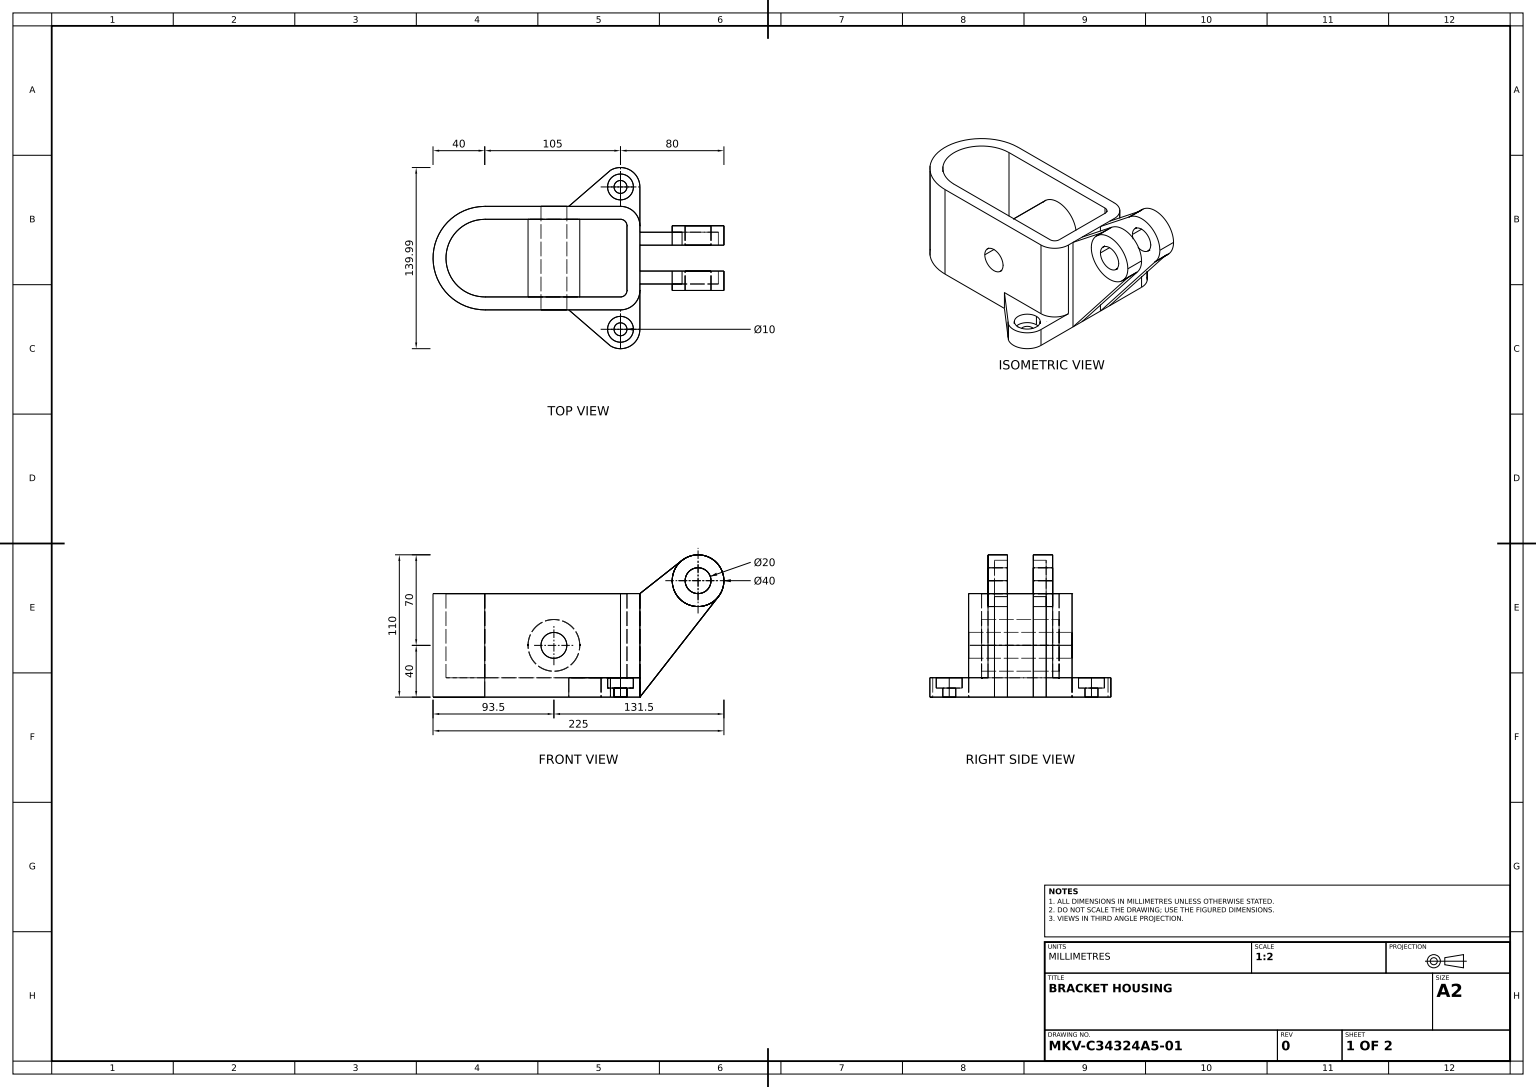
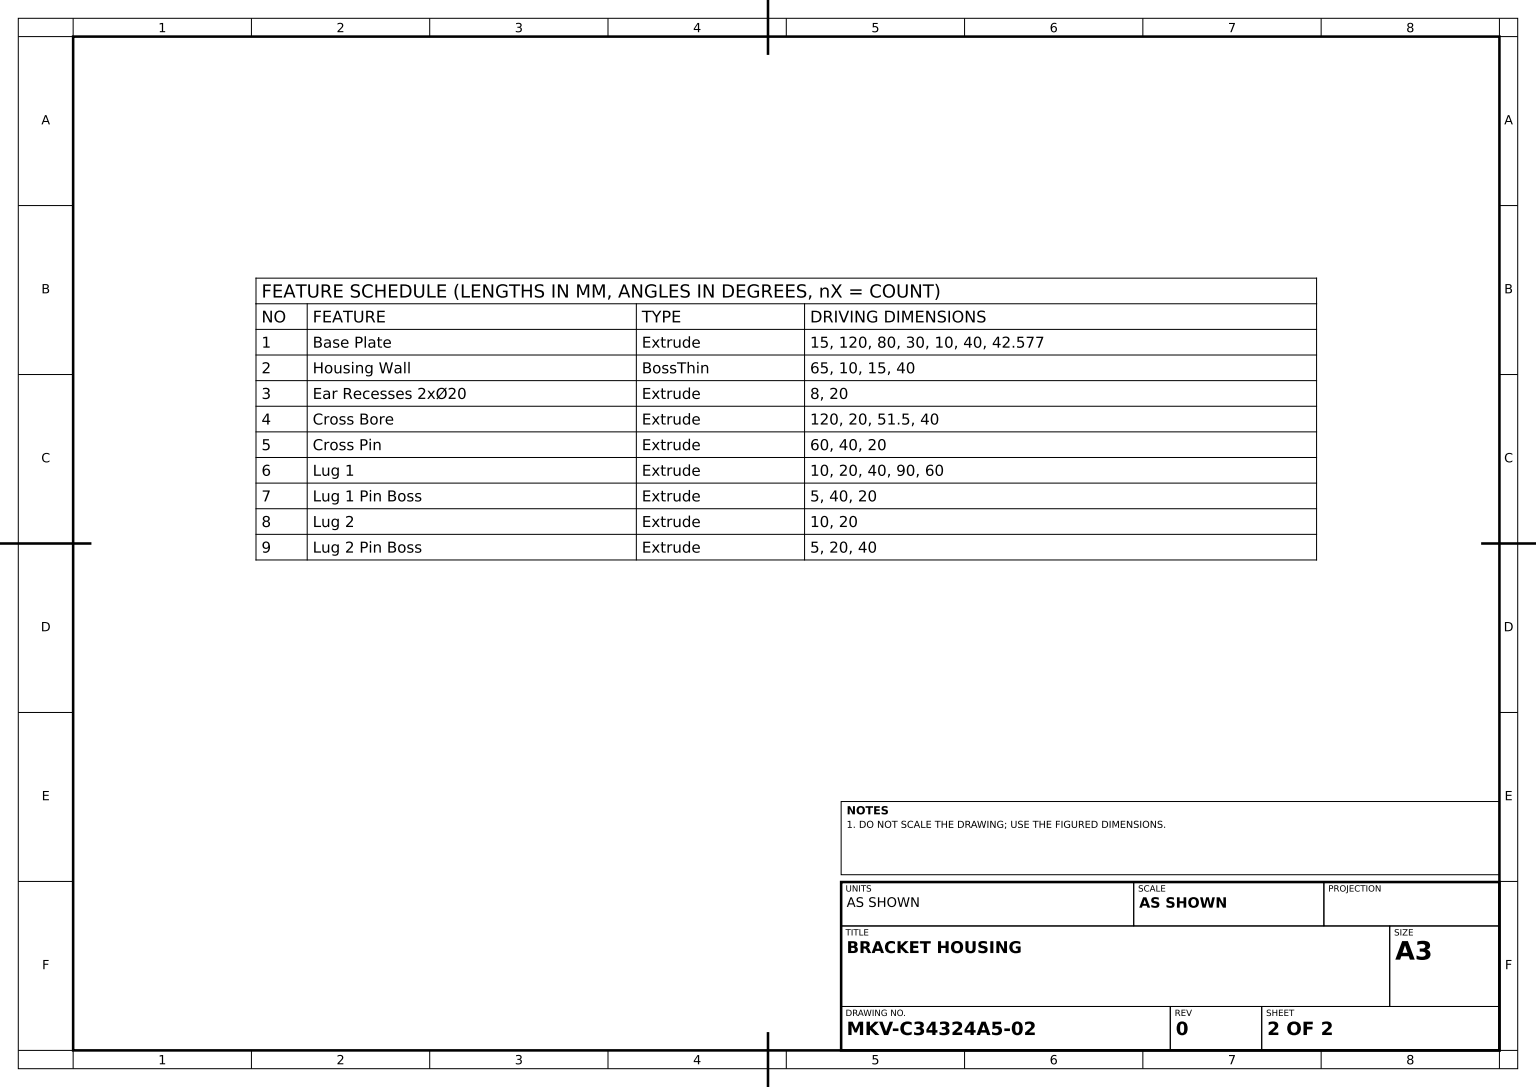
SolidWorks part; units mm, degrees
material "Plain Carbon Steel"
ref_plane "Front Plane" through (0, 0, 0) normal (0, 0, 1) x (1, 0, 0)
ref_plane "Top Plane" through (0, 0, 0) normal (0, 1, 0) x (1, 0, 0)
ref_plane "Right Plane" through (0, 0, 0) normal (1, 0, 0) x (0, 0, -1)
sketch "Base Plate Sketch" plane through (0, 0, 0) normal (0, 1, 0) x (1, 0, 0)
  line L0 (60, 55) -> (60, 40)
  line L1 (-60, -40) -> (45, -40)
  line L3 (-60, 40) -> (45, 40)
  line L4 (60, -25) -> (60, 25)
  line L5 (-60, -40) -> (60, 40) construction
  line L6 (-60, 40) -> (60, -40) construction
  line L7 (60, -40) -> (60, -55)
  line L8 (5, 40) -> (37.2247, 67.8275)
  line L9 (60, -25) -> (60, -40)
  line L10 (5, -40) -> (37.2247, -67.8275)
  line L11 (60, 40) -> (60, 25)
  circle A0 centre (45, -55) radius 5
  arc A1 (33.4419, -64.5609) -> (60, -55) centre (45, -55) ccw
  circle A2 centre (45, 55) radius 5
  arc A3 (60, 55) -> (33.4419, 64.5609) centre (45, 55) ccw
  arc A4 (-60, 40) -> (-60, -40) centre (-60, 0) ccw
  arc A5 (45, 40) -> (60, 25) centre (45, 25) cw
  arc A6 (45, -40) -> (60, -25) centre (45, -25) ccw
  point P0 (0, 0)
  dimension "D3" = 30
  dimension "D4" = 10
  dimension "D5" = 30
  dimension "D6" = 10
  dimension "D13" = 15
  dimension "D1" = 120
  dimension "D2" = 80
  dimension "D7" = 15
  dimension "D8" = 15
  dimension "D9" = 15
  dimension "D10" = 15
  dimension "D11" = 40
  dimension "D12" = 40
  dimension "D14" = 42.577
extrude "Base Plate" add sketch "Base Plate Sketch" along normal blind 15 contours L1 A6 L4 A5 L3 A4 | A6 L1 L10 A1 L7 L9 A0 | L3 A5 L11 L0 A3 L8 A2
sketch "Housing Wall Sketch" plane through (0, 15, 0) normal (0, 1, 0) x (1, 0, 0)
  line L0 (60, -55) -> (60, 55) construction
  line L1 (-60, -40) -> (45, -40)
  line L3 (-60, 40) -> (45, 40)
  line L4 (60, -25) -> (60, 25)
  line L5 (-60, -40) -> (60, 40) construction
  line L6 (-60, 40) -> (60, -40) construction
  arc A0 (-60, 40) -> (-60, -40) centre (-60, 0) ccw
  arc A1 (45, -40) -> (60, -25) centre (45, -25) ccw
  arc A2 (45, 40) -> (60, 25) centre (45, 25) cw
  point P0 (0, 0)
  dimension "D1" = 15
  dimension "D2" = 40
extrude "Housing Wall" add sketch "Housing Wall Sketch" along normal blind 65 thin thin type one direction reverse wall 10
sketch "Ear Recesses Sketch" plane through (0, 15, 0) normal (0, 1, 0) x (1, 0, 0)
  circle A0 centre (45, -55) radius 10
  circle A1 centre (45, 55) radius 10
  dimension "D1" = 20
  dimension "D2" = 20
extrude "Ear Recesses 2xØ20" cut sketch "Ear Recesses Sketch" against normal blind 8
sketch "Cross Bore Sketch" plane through (0, 0, 40) normal (0, 0, 1) x (1, 0, 0)
  line L2 (45, 80) -> (45, 15) construction
  line L3 (-60, 0) -> (5, 0) construction
  circle A0 centre (-6.5, 40) radius 10
  dimension "D1" = 20
  dimension "D2" = 51.5
  dimension "D3" = 40
extrude "Cross Bore" cut sketch "Cross Bore Sketch" against normal blind 120
sketch "Cross Pin Sketch" plane through (0, 0, -30) normal (0, 0, 1) x (1, 0, 0)
  circle A0 centre (-6.5, 40) radius 10
  circle A1 centre (-6.5, 40) radius 20
  dimension "D1" = 40
  dimension "D2" = 20
extrude "Cross Pin" add sketch "Cross Pin Sketch" along normal blind 60
ref_plane "Lug 1 Plane" through (0, 0, 10) normal (0, 0, 1) x (1, 0, 0)
sketch "Lug 1 Sketch" plane through (0, 0, 10) normal (0, 0, 1) x (1, 0, 0)
  line L0 (37.2247, 0) -> (60, 0) construction
  line L1 (45, 80) -> (45, 15) construction
  line L2 (60, 80) -> (92.6204, 105.7081)
  line L3 (60, 80) -> (60, 0)
  line L4 (60, 0) -> (120.7539, 77.6786)
  circle A0 centre (105, 90) radius 10
  circle A1 centre (105, 90) radius 20
  dimension "D1" = 20
  dimension "D2" = 40
  dimension "D3" = 90
  dimension "D4" = 60
extrude "Lug 1" add sketch "Lug 1 Sketch" along normal blind 10 contours A1 L2 L3 L4 | A1 A0
sketch "Lug 1 Pin Boss Sketch" plane through (0, 0, 20) normal (0, 0, 1) x (1, 0, 0)
  circle A0 centre (105, 90) radius 10
  circle A1 centre (105, 90) radius 20
  dimension "D1" = 40
  dimension "D2" = 20
extrude "Lug 1 Pin Boss" add sketch "Lug 1 Pin Boss Sketch" along normal blind 5
ref_plane "Lug 2 Plane" through (0, 0, -10) normal (0, 0, 1) x (1, 0, 0)
sketch "Lug 2 Sketch" plane through (0, 0, -10) normal (0, 0, 1) x (1, 0, 0)
  line L0 (92.6204, 105.7081) -> (60, 80)
  line L1 (60, 80) -> (60, 0)
  line L2 (60, 0) -> (120.7539, 77.6786)
  circle A0 centre (105, 90) radius 10
  circle A1 centre (105, 90) radius 20
  dimension "D1" = 20
extrude "Lug 2" add sketch "Lug 2 Sketch" against normal blind 10 contours A1 L0 L1 L2 | A1 A0
sketch "Lug 2 Pin Boss Sketch" plane through (0, 0, -20) normal (0, 0, -1) x (-1, 0, 0)
  circle A0 centre (-105, 90) radius 10
  circle A1 centre (-105, 90) radius 20
  dimension "D1" = 20
  dimension "D2" = 40
extrude "Lug 2 Pin Boss" add sketch "Lug 2 Pin Boss Sketch" along normal blind 5
